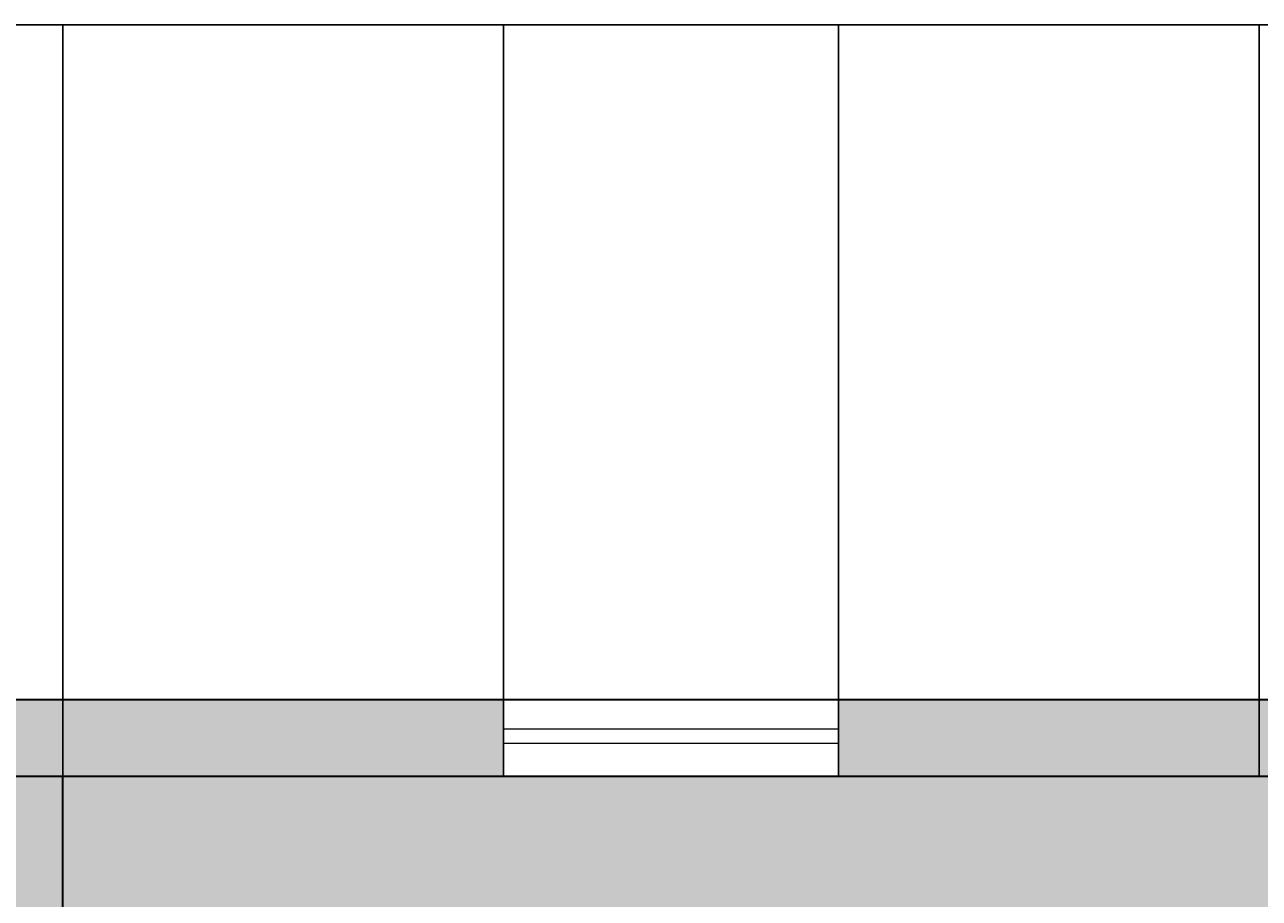
# Model space of a CAD drawing. Units: millimetres. Extents: x -229 to 16545, y -10488 to 4272.
# Tile 12 of 29: x 5862 to 9556, y 1656 to 4272. Entities that reach past the tile are written whole.
import ezdxf

# ---------------------------------------------------------------- set-up
doc = ezdxf.new("R2010")
doc.units = ezdxf.units.MM
for name, color, linetype, lineweight in [('A-ANNO-DIMS', 2, 'Continuous', 18), ('A-GLAZ', 4, 'Continuous', 18), ('A-WALL', 7, 'Continuous', 35)]:
    doc.layers.add(name, color=color, linetype=linetype, lineweight=lineweight)
doc.layers.add('A-FLOR-PATT', color=254, linetype='Continuous', lineweight=13, true_color=0xfeeab9)
doc.layers.add('A-WALL-PATT', color=18, linetype='Continuous', lineweight=13, true_color=0x000000)
doc.styles.get("Standard").update_dxf_attribs({"font": 'arial.ttf'})
doc.dimstyles.get("Standard").update_dxf_attribs({"dimtxt": 0.18, "dimasz": 0.18, "dimexe": 0.18, "dimexo": 0.0625, "dimgap": 0.09, "dimtad": 0, "dimtih": 1, "dimtoh": 1, "dimdec": 4, "dimzin": 0, "dimdsep": 46, "dimtxsty": 'Standard', "dimcen": 0.09, "dimadec": 0, "dimazin": 0, "dimtfac": 1, "dimtdec": 4, "dimtofl": 0, "dimtmove": 0, "dimatfit": 3, "dimfxl": 1, "dimtolj": 1, "dimtzin": 0, "dimarcsym": 0})

# ---------------------------------------------------------------- blocks, each defined once
blk = doc.blocks.new('*D45')
at = {"layer": 'A-ANNO-DIMS', "color": 0, "lineweight": -2, "transparency": 16777216}
for p, q in [((2015.9, 2251.8), (2015.9, 4271.7)), ((2016.1, 4271.5), (8015.5, 4271.5)), ((14015.8, 4271.5), (8016.4, 4271.5)), ((14015.9, 2251.8), (14015.9, 4271.7))]:
    blk.add_line(p, q, dxfattribs=at)
at = {"layer": 'A-ANNO-DIMS', "color": 0, "transparency": 16777216}
for points in [[(2016.1, 4271.5), (2016.1, 4271.4), (2015.9, 4271.5)], [(14015.8, 4271.5), (14015.8, 4271.4), (14015.9, 4271.5)]]:
    blk.add_solid(points, dxfattribs=at)
at = {"layer": 'Defpoints', "color": 0, "transparency": 16777216}
for p in [(14015.9, 4271.5), (2015.9, 2251.7), (14015.9, 2251.7)]:
    blk.add_point(p, dxfattribs=at)
at = {"layer": 'A-ANNO-DIMS', "color": 0, "transparency": 16777216, "insert": (8015.9, 4271.5), "char_height": 0.18, "attachment_point": 5}
blk.add_mtext('\\A1;12000', dxfattribs=at)
blk = doc.blocks.new('*D51')
at = {"layer": 'A-ANNO-DIMS', "color": 0, "lineweight": -2, "transparency": 16777216}
for p, q in [((5975.9, 2021.8), (5975.9, 4271.7)), ((5976.1, 4271.5), (7765.6, 4271.5)), ((9555.8, 4271.5), (7766.3, 4271.5)), ((9555.9, 2021.8), (9555.9, 4271.7))]:
    blk.add_line(p, q, dxfattribs=at)
at = {"layer": 'A-ANNO-DIMS', "color": 0, "transparency": 16777216}
for points in [[(5976.1, 4271.5), (5976.1, 4271.4), (5975.9, 4271.5)], [(9555.8, 4271.5), (9555.8, 4271.4), (9555.9, 4271.5)]]:
    blk.add_solid(points, dxfattribs=at)
at = {"layer": 'Defpoints', "color": 0, "transparency": 16777216}
for p in [(9555.9, 4271.5), (5975.9, 2021.7), (9555.9, 2021.7)]:
    blk.add_point(p, dxfattribs=at)
at = {"layer": 'A-ANNO-DIMS', "color": 0, "transparency": 16777216, "insert": (7765.9, 4271.5), "char_height": 0.18, "attachment_point": 5}
blk.add_mtext('\\A1;3580', dxfattribs=at)
blk = doc.blocks.new('*D71')
at = {"layer": 'A-ANNO-DIMS', "color": 0, "lineweight": -2, "transparency": 16777216}
for p, q in [((5975.9, 2021.8), (5975.9, 4271.7)), ((5976.1, 4271.5), (6634.7, 4271.5)), ((7294.2, 4271.5), (6635.6, 4271.5)), ((7294.4, 2021.8), (7294.4, 4271.7))]:
    blk.add_line(p, q, dxfattribs=at)
at = {"layer": 'A-ANNO-DIMS', "color": 0, "transparency": 16777216}
for points in [[(5976.1, 4271.5), (5976.1, 4271.4), (5975.9, 4271.5)], [(7294.2, 4271.5), (7294.2, 4271.4), (7294.4, 4271.5)]]:
    blk.add_solid(points, dxfattribs=at)
at = {"layer": 'Defpoints', "color": 0, "transparency": 16777216}
for p in [(7294.4, 4271.5), (5975.9, 2021.7), (7294.4, 2021.7)]:
    blk.add_point(p, dxfattribs=at)
at = {"layer": 'A-ANNO-DIMS', "color": 0, "transparency": 16777216, "insert": (6635.2, 4271.5), "char_height": 0.18, "attachment_point": 5}
blk.add_mtext('\\A1;1318.5', dxfattribs=at)
blk = doc.blocks.new('*D72')
at = {"layer": 'A-ANNO-DIMS', "color": 0, "lineweight": -2, "transparency": 16777216}
for p, q in [((7294.4, 2021.8), (7294.4, 4271.7)), ((7294.6, 4271.5), (7795.1, 4271.5)), ((8296.6, 4271.5), (7796, 4271.5)), ((8296.8, 2021.8), (8296.8, 4271.7))]:
    blk.add_line(p, q, dxfattribs=at)
at = {"layer": 'A-ANNO-DIMS', "color": 0, "transparency": 16777216}
for points in [[(7294.6, 4271.5), (7294.6, 4271.4), (7294.4, 4271.5)], [(8296.6, 4271.5), (8296.6, 4271.4), (8296.8, 4271.5)]]:
    blk.add_solid(points, dxfattribs=at)
at = {"layer": 'Defpoints', "color": 0, "transparency": 16777216}
for p in [(8296.8, 4271.5), (7294.4, 2021.7), (8296.8, 2021.7)]:
    blk.add_point(p, dxfattribs=at)
at = {"layer": 'A-ANNO-DIMS', "color": 0, "transparency": 16777216, "insert": (7795.6, 4271.5), "char_height": 0.18, "attachment_point": 5}
blk.add_mtext('\\A1;1002.3', dxfattribs=at)
blk = doc.blocks.new('*D85')
at = {"layer": 'A-ANNO-DIMS', "color": 0, "lineweight": -2, "transparency": 16777216}
for p, q in [((5745.9, 755.6), (5745.9, 4271.7)), ((5746.1, 4271.5), (5860.6, 4271.5)), ((5975.8, 4271.5), (5861.2, 4271.5)), ((5975.9, 755.6), (5975.9, 4271.7))]:
    blk.add_line(p, q, dxfattribs=at)
at = {"layer": 'A-ANNO-DIMS', "color": 0, "transparency": 16777216}
for points in [[(5746.1, 4271.5), (5746.1, 4271.4), (5745.9, 4271.5)], [(5975.8, 4271.5), (5975.8, 4271.4), (5975.9, 4271.5)]]:
    blk.add_solid(points, dxfattribs=at)
at = {"layer": 'Defpoints', "color": 0, "transparency": 16777216}
for p in [(5975.9, 4271.5), (5745.9, 755.5), (5975.9, 755.5)]:
    blk.add_point(p, dxfattribs=at)
at = {"layer": 'A-ANNO-DIMS', "color": 0, "transparency": 16777216, "insert": (5860.9, 4271.5), "char_height": 0.18, "attachment_point": 5}
blk.add_mtext('\\A1;230', dxfattribs=at)
blk = doc.blocks.new('*D100')
at = {"layer": 'A-ANNO-DIMS', "color": 0, "lineweight": -2, "transparency": 16777216}
for p, q in [((7294.4, 2021.7), (-228.8, 2021.7)), ((-228.7, 2021.5), (-228.7, 1688.2)), ((-228.7, 1354.6), (-228.7, 1687.9)), ((8024.8, 1354.4), (-228.8, 1354.4))]:
    blk.add_line(p, q, dxfattribs=at)
at = {"layer": 'A-ANNO-DIMS', "color": 0, "transparency": 16777216}
for points in [[(-228.7, 2021.5), (-228.6, 2021.5), (-228.7, 2021.7)], [(-228.7, 1354.6), (-228.6, 1354.6), (-228.7, 1354.4)]]:
    blk.add_solid(points, dxfattribs=at)
at = {"layer": 'Defpoints', "color": 0, "transparency": 16777216}
for p in [(7294.4, 2021.7), (-228.7, 1354.4), (8024.9, 1354.4)]:
    blk.add_point(p, dxfattribs=at)
at = {"layer": 'A-ANNO-DIMS', "color": 0, "transparency": 16777216, "insert": (-228.7, 1688.1), "char_height": 0.18, "attachment_point": 5}
blk.add_mtext('\\A1;667.3', dxfattribs=at)

msp = doc.modelspace()

# ---------------------------------------------------------------- hatches: boundary and pattern name
at = {"layer": 'A-FLOR-PATT', "transparency": 33554592}
h = msp.add_hatch(color=256, dxfattribs=at)
h.dxf.hatch_style = 1
h.paths.add_polyline_path([(7975.933, -5325.772), (7943.121, -5325.772), (7943.121, -4576.49, 0.40145271), (7225.933, -5325.772, 0.40145271), (6508.746, -4576.49), (6508.746, -5325.772), (6475.933, -5325.772), (6475.933, -5438.272), (5975.933, -5438.272), (5975.933, -7267.724), (5975.933, -7438.272), (6478.619, -7438.272), (6463.448, -7355.919), (6464.88, -7356.837), (6463.849, -7358.097), (6478.619, -7438.272), (6610.327, -7438.272), (6632.656, -7409.564), (6632.525, -7406.967), (6634.208, -7407.569), (6619.273, -7426.77), (6654.466, -7438.272), (7610.517, -7438.272), (7607.41, -7421.409), (7608.842, -7422.327), (7607.812, -7423.587), (7610.517, -7438.272), (7975.933, -7438.272)])
h.paths.add_polyline_path([(13785.933, -1208.272), (9555.933, -1208.272), (9555.933, -961.785), (9705.933, -961.785), (9705.933, -918.035), (10704.976, -918.035, 0.40145271), (9705.933, 38.215), (9555.933, 38.215), (9555.933, 2021.728), (5975.933, 2021.728), (5975.933, 755.492), (5745.933, 755.492), (5745.933, 1427.266), (2918.813, 1427.266), (2918.813, -492.942), (5013.319, -492.942), (5013.319, -978.272), (5745.933, -978.272), (5745.933, -397.513), (5975.933, -397.513), (5975.933, -1208.272), (4560.933, -1208.272), (4560.933, -1265.772), (4448.433, -1265.772), (4448.433, -1298.585), (4445.933, -1298.585), (3699.151, -1298.585, 0.40145271), (4448.433, -2015.772), (4560.933, -2015.772), (4560.933, -2384.177), (5745.933, -2384.177), (5799.402, -2384.177), (5799.402, -4518.272), (5975.933, -4518.272), (5975.933, -5208.272), (6475.933, -5208.272), (6475.933, -4575.772), (6508.746, -4575.772), (6508.746, -4576.49, -0.35647263), (7216.672, -5208.272), (7235.194, -5208.272, -0.35647263), (7943.121, -4576.49), (7943.121, -4575.772), (7975.933, -4575.772), (7975.933, -5208.272), (11176.247, -5208.272), (11159.44, -5191.465), (10520.768, -5191.465), (10520.768, -4888.936), (10571.19, -4888.936), (10571.19, -4872.129), (10772.876, -4872.129), (10772.876, -4888.936), (10789.683, -4888.936), (10789.683, -4872.129), (10991.368, -4872.129), (10991.368, -4888.936), (11041.79, -4888.936), (11041.79, -4872.129), (11058.597, -4872.129, -0.09090909), (11428.354, -4872.129), (11445.162, -4872.129), (11445.162, -4888.936), (11529.197, -4888.936), (11529.197, -5191.465), (11327.512, -5191.465), (11310.704, -5208.272), (13785.933, -5208.272)])
h.paths.add_polyline_path([(11047.216, -1630.944, -1), (11402.816, -1630.944, -1)], flags=16)
h.paths.add_polyline_path([(11148.816, -1630.944), (11225.016, -1554.744), (11301.216, -1630.944), (11225.016, -1707.144)], flags=0)
h.paths.add_polyline_path([(11199.616, -1630.944, -1), (11250.416, -1630.944, -1)], flags=0)
h.paths.add_polyline_path([(11588.751, -2096.259), (11588.751, -1543.254, -0.26666697), (12864.918, -1543.254), (12864.918, -2096.259), (12737.302, -2096.259), (12737.302, -2063.121), (11716.368, -2063.121), (11716.368, -2096.259)], flags=16)
h.paths.add_polyline_path([(12012.696, -2489.42), (12600.997, -2489.42), (12600.997, -3666.022), (12012.696, -3666.022)], flags=16)
h.paths.add_polyline_path([(12176.41, -3599.403), (12174.938, -3609.076), (12173.789, -3618.819), (12173.09, -3628.559), (12172.973, -3638.221), (12173.89, -3652.852), (12175.008, -3657.025), (12172.909, -3643.473), (12173.142, -3624.297), (12175.386, -3605.273)], flags=0)
h.paths.add_polyline_path([(8026.289, -286.944), (7737.703, -287.19), (7734.87, -269.156), (8029.092, -268.905)], flags=16)
h.paths.add_polyline_path([(7733.453, -260.139), (7710.784, -115.865), (7557.191, -115.996), (7556.999, 109.744), (7412.687, 132.166), (7412.433, 429.206), (7556.707, 451.876), (7556.568, 614.769), (7412.256, 637.19), (7412.003, 934.231), (7556.276, 956.9), (7556.084, 1182.639), (7709.677, 1182.77), (7732.099, 1327.082), (8029.14, 1327.335), (8051.808, 1183.062), (8205.401, 1183.192), (8205.594, 957.454), (8349.906, 935.031), (8350.159, 637.99), (8205.885, 615.322), (8206.024, 452.43), (8350.336, 430.006), (8350.59, 132.965), (8206.316, 110.298), (8206.509, -115.442), (8052.916, -115.573), (8030.493, -259.885)], flags=16)
h.paths.add_polyline_path([(12261.416, -3475.554), (12262.632, -3486.776), (12264.032, -3497.007), (12265.554, -3506.365), (12267.136, -3514.968), (12268.719, -3522.935), (12271.304, -3535.59), (12273.606, -3548.078), (12275.271, -3561.064), (12275.93, -3574.938), (12275.325, -3590.3), (12273.425, -3607.964), (12270.795, -3625.658), (12268.066, -3641.063), (12266.318, -3649.679), (12265.456, -3653.626), (12263.984, -3659.846), (12264.032, -3659.566), (12264.342, -3658.241), (12264.807, -3656.37), (12265.456, -3653.626), (12266.318, -3649.679), (12267.409, -3644.302), (12268.668, -3637.664), (12270.019, -3630.037), (12271.384, -3621.695), (12272.69, -3612.908), (12273.857, -3603.948), (12274.81, -3595.088), (12275.47, -3586.601), (12275.782, -3578.689), (12275.757, -3571.292), (12275.423, -3564.275), (12274.816, -3557.512), (12273.964, -3550.872), (12272.896, -3544.224), (12271.645, -3537.439), (12270.24, -3530.385), (12267.543, -3517.181), (12264.612, -3501.247), (12261.849, -3481.059)], flags=0)
h.paths.add_polyline_path([(12332.136, -3408.03), (12333.483, -3416.79), (12335.077, -3424.54), (12336.915, -3431.355), (12338.991, -3437.32), (12341.266, -3442.55), (12343.694, -3447.166), (12346.229, -3451.292), (12348.826, -3455.051), (12351.438, -3458.563), (12357.476, -3466.491), (12363.61, -3476.575), (12368.309, -3489.762), (12369.929, -3503.427), (12369.842, -3516.511), (12368.43, -3530.867), (12365.816, -3545.835), (12362.382, -3559.786), (12360.968, -3564.487), (12363.063, -3557.021), (12364.898, -3549.566), (12366.473, -3542.077), (12367.773, -3534.631), (12368.781, -3527.301), (12369.483, -3520.162), (12369.863, -3513.291), (12369.906, -3506.759), (12369.599, -3500.643), (12368.93, -3494.999), (12367.924, -3489.796), (12366.61, -3484.994), (12365.024, -3480.542), (12363.19, -3476.399), (12361.141, -3472.516), (12358.909, -3468.847), (12356.525, -3465.347), (12354.02, -3461.954), (12351.438, -3458.563), (12345.462, -3450.529), (12339.923, -3439.996), (12335.85, -3428.296), (12332.68, -3412.888)], flags=0)
h.paths.add_polyline_path([(12385.287, -3334.612), (12384.977, -3342.409), (12385.02, -3349.196), (12385.4, -3355.066), (12386.104, -3360.105), (12387.112, -3364.41), (12388.412, -3368.071), (12389.987, -3371.181), (12391.823, -3373.832), (12393.919, -3376.097), (12396.337, -3377.978), (12399.153, -3379.462), (12402.445, -3380.531), (12406.289, -3381.172), (12410.758, -3381.371), (12415.935, -3381.106), (12421.893, -3380.368), (12428.658, -3379.159), (12436.069, -3377.55), (12443.907, -3375.635), (12451.961, -3373.505), (12460.015, -3371.254), (12467.853, -3368.971), (12475.263, -3366.749), (12482.029, -3364.68), (12491.877, -3361.657), (12497.701, -3360.107), (12501.639, -3359.288), (12510.135, -3358.326), (12519.662, -3365.412), (12524.243, -3378.911), (12523.764, -3390.7), (12520.746, -3401.577), (12514.248, -3415.634), (12511.518, -3420.418), (12515.856, -3412.154), (12519.153, -3405.024), (12521.516, -3398.804), (12523.049, -3393.276), (12523.865, -3388.212), (12524.059, -3383.441), (12523.7, -3378.958), (12522.853, -3374.815), (12521.576, -3371.054), (12519.931, -3367.722), (12517.982, -3364.865), (12515.786, -3362.529), (12513.405, -3360.758), (12510.877, -3359.588), (12508.136, -3358.982), (12505.086, -3358.897), (12501.639, -3359.288), (12497.701, -3360.107), (12493.183, -3361.309), (12487.988, -3362.851), (12476.403, -3366.408), (12463.335, -3370.326), (12447.372, -3374.788), (12431.759, -3378.604), (12418.504, -3380.974), (12405.811, -3381.624), (12394.725, -3378.025), (12388.039, -3368.367), (12385.583, -3357.877), (12384.826, -3346.204), (12385.428, -3331.059), (12385.953, -3325.719)], flags=0)
h.paths.add_polyline_path([(7880.016, 1173.969), (7880.373, 1175.495), (7880.433, 1175.851), (7879.484, 1171.818)], flags=0)
h.paths.add_polyline_path([(7802.33, 874.962), (7800.771, 885.032), (7798.932, 893.941), (7796.811, 901.774), (7794.419, 908.63), (7791.798, 914.639), (7789.002, 919.945), (7786.083, 924.686), (7783.093, 929.005), (7780.087, 933.043), (7774.996, 939.717), (7768.406, 949.37), (7762.174, 963.427), (7759.342, 978.002), (7758.629, 991.888), (7759.492, 1007.928), (7761.801, 1025.496), (7765.392, 1044.035), (7766.625, 1049.048), (7764.522, 1039.543), (7762.719, 1030.232), (7761.232, 1021.168), (7760.08, 1012.405), (7759.28, 1003.994), (7758.849, 995.988), (7758.806, 988.44), (7759.167, 981.404), (7759.942, 974.914), (7761.104, 968.936), (7762.617, 963.414), (7764.448, 958.299), (7766.559, 953.535), (7768.918, 949.073), (7771.487, 944.856), (7774.232, 940.835), (7777.115, 936.938), (7782.377, 930.041), (7787.845, 922.139), (7793.348, 911.698), (7798.042, 898.247), (7801.702, 880.527)], flags=0)
h.paths.add_polyline_path([(12519.068, -3228.534), (12519.615, -3236.235), (12520.529, -3242.343), (12521.78, -3247.103), (12523.337, -3250.758), (12525.171, -3253.556), (12527.248, -3255.709), (12529.522, -3257.296), (12531.95, -3258.361), (12534.486, -3258.949), (12537.082, -3259.11), (12539.694, -3258.888), (12542.277, -3258.329), (12544.781, -3257.478), (12547.173, -3256.388), (12549.46, -3255.129), (12550.455, -3254.517), (12555.825, -3251.109), (12557.835, -3249.942), (12565.181, -3246.404), (12574.565, -3253.032), (12576.931, -3265.022), (12576.627, -3277.425), (12575.416, -3290.819), (12574.851, -3295.392), (12575.708, -3287.593), (12576.322, -3280.806), (12576.688, -3274.939), (12576.812, -3269.899), (12576.688, -3265.593), (12576.322, -3261.932), (12575.708, -3258.822), (12574.851, -3256.172), (12573.753, -3253.905), (12572.439, -3252.005), (12570.943, -3250.474), (12569.293, -3249.309), (12567.523, -3248.513), (12565.658, -3248.083), (12563.732, -3248.022), (12561.777, -3248.328), (12559.814, -3248.989), (12557.835, -3249.942), (12555.825, -3251.109), (12553.77, -3252.413), (12551.652, -3253.78), (12549.46, -3255.129), (12543.167, -3258.594), (12532.661, -3259.485), (12524.685, -3253.923), (12520.949, -3245.152), (12519.138, -3233.042)], flags=0)
h.paths.add_polyline_path([(7741.293, 790.501), (7741.641, 799.467), (7741.584, 807.269), (7741.141, 814.015), (7740.329, 819.809), (7739.165, 824.757), (7737.667, 828.966), (7735.853, 832.541), (7733.74, 835.586), (7731.348, 838.188), (7728.71, 840.348), (7725.861, 842.052), (7722.836, 843.28), (7719.671, 844.015), (7716.4, 844.237), (7713.06, 843.932), (7709.684, 843.081), (7706.304, 841.686), (7702.923, 839.834), (7699.543, 837.629), (7696.164, 835.178), (7692.784, 832.585), (7684.718, 826.315), (7675.609, 820.63), (7664.001, 817.274), (7654.105, 821.884), (7647.171, 832.02), (7644.191, 846.522), (7646.321, 860.288), (7647.49, 864.223), (7645.946, 857.865), (7645.046, 852.044), (7644.827, 846.557), (7645.243, 841.404), (7646.221, 836.642), (7647.693, 832.318), (7649.587, 828.489), (7651.832, 825.206), (7654.359, 822.523), (7657.097, 820.49), (7659.984, 819.145), (7662.993, 818.452), (7666.108, 818.357), (7669.311, 818.809), (7672.583, 819.755), (7675.908, 821.139), (7679.268, 822.913), (7682.645, 825.021), (7686.025, 827.401), (7689.404, 829.958), (7692.784, 832.585), (7700.505, 838.509), (7709.871, 843.64), (7721.436, 844.698), (7733.277, 837.617), (7739.571, 825.214), (7741.557, 811.049), (7741.669, 795.575)], flags=0)
h.paths.add_polyline_path([(8377.641, 137.216), (8359.607, 134.382), (8359.356, 428.605), (8377.395, 425.802)], flags=16)
h.paths.add_polyline_path([(7650.715, 668.465), (7650.08, 677.319), (7649.023, 684.34), (7647.579, 689.811), (7645.785, 694.012), (7643.675, 697.228), (7641.286, 699.7), (7638.669, 701.521), (7635.876, 702.744), (7632.96, 703.419), (7629.974, 703.601), (7626.971, 703.344), (7624.004, 702.697), (7621.125, 701.717), (7618.375, 700.462), (7615.749, 699.013), (7614.561, 698.279), (7608.435, 694.382), (7606.125, 693.04), (7598.981, 689.594), (7589.669, 693.773), (7585.26, 702.856), (7584.221, 713.11), (7584.49, 724.584), (7585.863, 739.937), (7586.518, 745.277), (7585.539, 736.31), (7584.841, 728.507), (7584.424, 721.761), (7584.288, 715.966), (7584.433, 711.016), (7584.86, 706.807), (7585.567, 703.231), (7586.556, 700.186), (7587.821, 697.58), (7589.332, 695.397), (7591.053, 693.637), (7592.951, 692.3), (7594.989, 691.385), (7597.132, 690.895), (7599.346, 690.826), (7601.594, 691.18), (7603.851, 691.943), (7606.125, 693.04), (7608.435, 694.382), (7610.797, 695.885), (7613.229, 697.458), (7620.475, 701.929), (7632.001, 704.44), (7643.476, 699.417), (7648.536, 687.571), (7650.63, 673.661)], flags=0)
h.paths.add_polyline_path([(7385.628, 136.37), (7385.382, 424.956), (7403.416, 427.789), (7403.667, 133.567)], flags=16)
h.paths.add_polyline_path([(12993.884, -2257.186), (12959.588, -2257.186), (12959.588, -2125.099), (13531.966, -2125.099, -0.19047621), (13531.966, -3974.321), (12959.588, -3974.321), (12959.588, -3842.233), (12993.884, -3842.233)], flags=16)
h.paths.add_polyline_path([(13413.486, -3313.884), (13413.486, -2785.535), (13562.885, -2785.535, -0.04962821), (13562.885, -3313.884)], flags=0)
h.paths.add_polyline_path([(8377.21, 642.241), (8359.176, 639.407), (8358.925, 933.629), (8376.964, 930.826)], flags=16)
h.paths.add_polyline_path([(13086.058, -1864.83), (13086.058, -1449.84), (13501.048, -1449.84), (13501.048, -1864.83)], flags=16)
h.paths.add_polyline_path([(13305.814, -1862.197), (13302.103, -1859.624), (13298.088, -1857.068), (13293.799, -1854.536), (13289.262, -1852.031), (13284.504, -1849.559), (13279.554, -1847.125), (13274.439, -1844.735), (13269.17, -1842.389), (13263.701, -1840.081), (13257.97, -1837.797), (13251.914, -1835.525), (13245.472, -1833.252), (13238.582, -1830.968), (13231.18, -1828.66), (13223.206, -1826.315), (13209.182, -1822.458), (13204.584, -1821.48), (13217.962, -1824.773), (13235.072, -1829.804), (13248.777, -1834.349), (13260.829, -1838.869), (13274.479, -1844.63), (13289.675, -1852.101), (13302.553, -1859.704)], flags=0)
h.paths.add_polyline_path([(13428.104, -1820.994), (13419.007, -1818.141), (13409.95, -1815.4), (13400.766, -1812.747), (13391.271, -1810.151), (13376.087, -1806.251), (13370.618, -1805.019), (13386.304, -1808.794), (13405.087, -1813.928), (13423.014, -1819.354)], flags=0)
h.paths.add_polyline_path([(7385.197, 641.395), (7384.951, 929.98), (7402.986, 932.814), (7403.236, 638.592)], flags=16)
h.paths.add_polyline_path([(13262.537, -1725.526), (13253.246, -1724.74), (13244.516, -1724.117), (13235.94, -1723.625), (13223.267, -1723.062), (13217.598, -1722.912), (13231.966, -1723.397), (13248.733, -1724.359), (13266.899, -1725.895), (13272.802, -1726.502)], flags=0)
h.paths.add_polyline_path([(13191.893, -1641.137), (13208.675, -1640.506), (13214.057, -1640.258), (13197.763, -1640.936)], flags=0)
h.paths.add_polyline_path([(13097.524, -1608.457), (13114.284, -1609.031), (13120.126, -1609.105), (13103.045, -1608.71)], flags=0)
h.paths.add_polyline_path([(13465.328, -1521.577), (13473.906, -1517.015), (13481.761, -1511.636), (13492.562, -1502.076), (13495.327, -1497.933), (13485.818, -1508.858), (13470.208, -1519.547)], flags=0)
h.paths.add_polyline_path([(13175.015, -1500.891), (13184.046, -1501.807), (13192.721, -1502.52), (13201.114, -1503.034), (13209.273, -1503.351), (13217.244, -1503.476), (13225.078, -1503.41), (13232.821, -1503.16), (13240.524, -1502.728), (13248.233, -1502.117), (13255.993, -1501.322), (13263.825, -1500.293), (13271.746, -1498.974), (13279.775, -1497.305), (13287.928, -1495.229), (13296.222, -1492.688), (13304.675, -1489.622), (13313.304, -1485.975), (13322.089, -1481.727), (13330.859, -1477.028), (13339.408, -1472.063), (13347.526, -1467.02), (13355.006, -1462.087), (13364.86, -1455.202), (13367.224, -1453.299), (13358.544, -1459.754), (13343.348, -1469.775), (13326.143, -1479.767), (13309.023, -1488.045), (13292.249, -1494.129), (13276.009, -1498.264), (13260.299, -1500.88), (13244.401, -1502.51), (13228.945, -1503.378), (13213.316, -1503.508), (13197.047, -1502.876), (13180.088, -1501.481)], flags=0)
h.paths.add_polyline_path([(7733.501, 1336.101), (7736.303, 1354.14), (8024.889, 1354.386), (8027.723, 1336.352)], flags=16)
at = {"layer": 'A-WALL-PATT'}
h = msp.add_hatch(color=256, dxfattribs=at)
h.dxf.hatch_style = 1
h.paths.add_polyline_path([(7294.425, 2163.983), (7294.425, 2251.728), (4412.722, 2251.728), (4412.722, 2166.741), (4412.722, 2122.457), (4412.722, 2021.728), (7294.425, 2021.728), (7294.425, 2119.698)])
h.paths.add_polyline_path([(11407.51, 2166.741), (11407.51, 2251.728), (8296.763, 2251.728), (8296.763, 2163.983), (8296.763, 2119.698), (8296.763, 2021.728), (11407.51, 2021.728), (11407.51, 2122.457)])
h.paths.add_polyline_path([(9785.933, 2021.728), (9555.933, 2021.728), (9555.933, 38.215), (9705.933, 38.215, -0.02002407), (9785.933, 35.01)])
h.paths.add_polyline_path([(14015.933, 2251.728), (12488.002, 2251.728), (12488.002, 2166.742), (12488.002, 2122.738), (12488.002, 2021.728), (13785.933, 2021.728), (13785.933, -2305.465), (13883.903, -2305.465), (13928.188, -2305.465), (14015.933, -2305.465)])
h.paths.add_polyline_path([(13785.933, -978.272), (9785.933, -978.272), (9785.933, -961.785), (9705.933, -961.785), (9555.933, -961.785), (9555.933, -1208.272), (13785.933, -1208.272)])
h.paths.add_polyline_path([(5975.933, 2021.728), (5745.933, 2021.728), (5745.933, 755.492), (5975.933, 755.492)])
h.paths.add_polyline_path([(2245.933, 2021.728), (3420.865, 2021.728), (3420.865, 2122.457), (3420.865, 2167.104), (3420.865, 2251.728), (2015.933, 2251.728), (2015.933, -3326.811), (2100.943, -3326.811), (2155.199, -3326.811), (2245.933, -3326.811)])
h.paths.add_polyline_path([(5975.933, -397.513), (5745.933, -397.513), (5745.933, -978.272), (2245.933, -978.272), (2245.933, -1208.272), (5975.933, -1208.272)])
h.paths.add_polyline_path([(12015.17, -5208.272), (7975.933, -5208.272), (7975.933, -5325.772), (7975.933, -5438.272), (7975.933, -5596.884), (8205.933, -5596.884), (8205.933, -5438.272), (12015.17, -5438.272), (12015.17, -5337.543), (12015.17, -5293.259)])
h.paths.add_polyline_path([(5975.933, -4518.272), (4567.83, -4518.272), (4567.83, -4603.259), (4567.83, -4647.543), (4567.83, -4748.272), (5745.933, -4748.272), (5745.933, -5438.272), (5975.933, -5438.272), (6475.933, -5438.272), (6475.933, -5325.772), (6475.933, -5208.272), (5975.933, -5208.272)])
h.paths.add_polyline_path([(3765.491, -4518.272), (2245.933, -4518.272), (2245.933, -4748.272), (3765.491, -4748.272), (3765.491, -4647.543), (3765.491, -4603.259)])

# ---------------------------------------------------------------- linework, layer by layer
at = {"layer": 'A-GLAZ'}
for p, q in [((7294.425, 2163.983), (7294.425, 2251.728)), ((8296.763, 2163.983), (8296.763, 2251.728)), ((7294.425, 2119.698), (7294.425, 2021.728)), ((8296.763, 2119.698), (8296.763, 2021.728))]:
    msp.add_line(p, q, dxfattribs=at)
msp.add_lwpolyline([(7294.425, 2163.983), (8296.763, 2163.983), (8296.763, 2119.698), (7294.425, 2119.698)], close=True, dxfattribs=at)
at = {"layer": 'A-WALL'}
for p, q in [((2015.933, 2251.728), (14015.933, 2251.728)), ((2245.933, 2021.728), (13785.933, 2021.728)), ((5975.933, 755.492), (5975.933, 2021.728))]:
    msp.add_line(p, q, dxfattribs=at)

# ---------------------------------------------------------------- dimensions: what is measured, and where the dimension line sits
at = {"layer": 'A-ANNO-DIMS'}
for base, p1, p2, override, picture, middle in [((14015.933, 4271.479), (2015.933, 2251.728), (14015.933, 2251.728), {"dimdec": 0, "dimlfac": 1, "dimrnd": 0, "dimzin": 0, "dimdsep": 46, "dimlunit": 2}, '*D45', (8015.933, 4271.479)), ((5975.933, 4271.479), (5745.933, 755.492), (5975.933, 755.492), {"dimdec": 0, "dimlfac": 1, "dimrnd": 0, "dimzin": 0, "dimdsep": 46, "dimlunit": 2}, '*D85', (5860.933, 4271.479)), ((9555.933, 4271.479), (5975.933, 2021.728), (9555.933, 2021.728), {"dimdec": 0, "dimlfac": 1, "dimrnd": 0, "dimzin": 0, "dimdsep": 46, "dimlunit": 2}, '*D51', (7765.933, 4271.479)), ((7294.425, 4271.479), (5975.933, 2021.728), (7294.425, 2021.728), {"dimdec": 1, "dimlfac": 1, "dimrnd": 0, "dimzin": 0, "dimdsep": 46, "dimlunit": 2}, '*D71', (6635.179, 4271.479)), ((8296.763, 4271.479), (7294.425, 2021.728), (8296.763, 2021.728), {"dimdec": 1, "dimlfac": 1, "dimrnd": 0, "dimzin": 0, "dimdsep": 46, "dimlunit": 2}, '*D72', (7795.594, 4271.479))]:
    dim = msp.add_linear_dim(base=base, p1=p1, p2=p2, dimstyle='Standard', override=override, dxfattribs=at)
    dim.commit()
    dim.dimension.update_dxf_attribs({"geometry": picture, "text_midpoint": middle})
dim = msp.add_linear_dim(base=(-228.657, 1354.386), p1=(7294.425, 2021.728), p2=(8024.889, 1354.386), angle=90, dimstyle='Standard', override={"dimdec": 1, "dimlfac": 1, "dimrnd": 0, "dimzin": 0, "dimdsep": 46, "dimlunit": 2}, dxfattribs=at)
dim.commit()
dim.dimension.update_dxf_attribs({"geometry": '*D100', "text_midpoint": (-228.657, 1688.057)})

doc.saveas('drawing.dxf')
